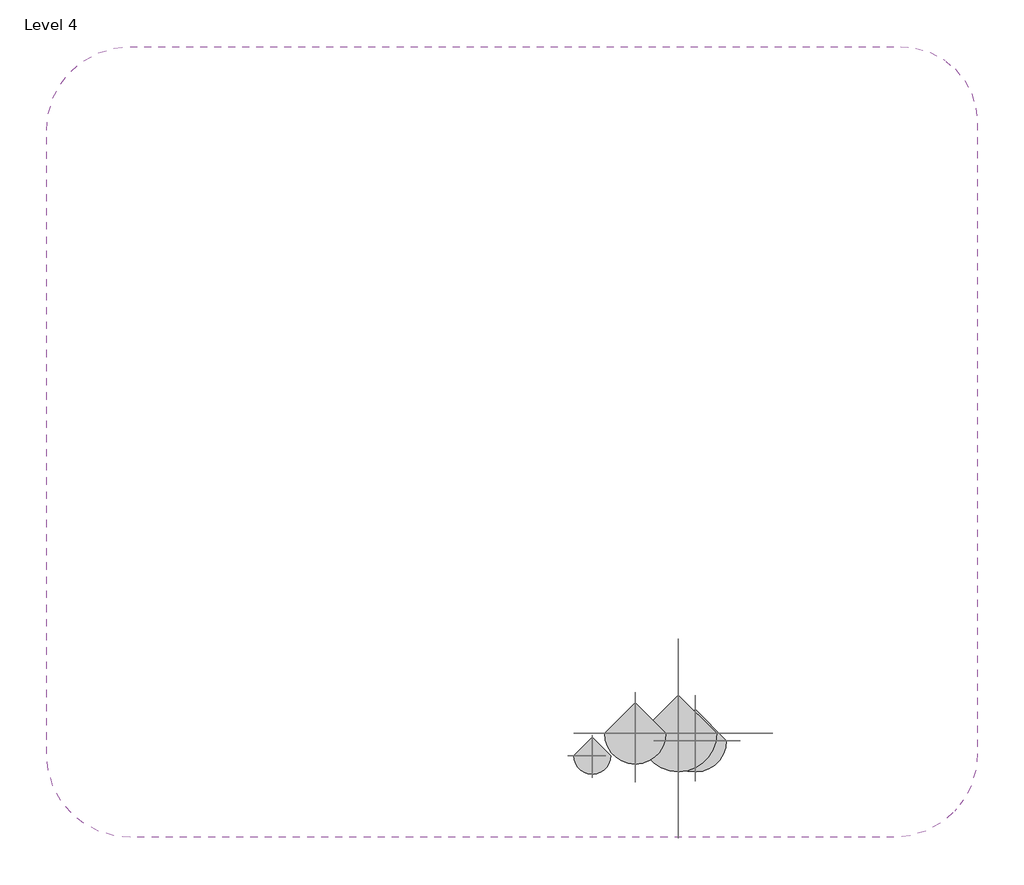
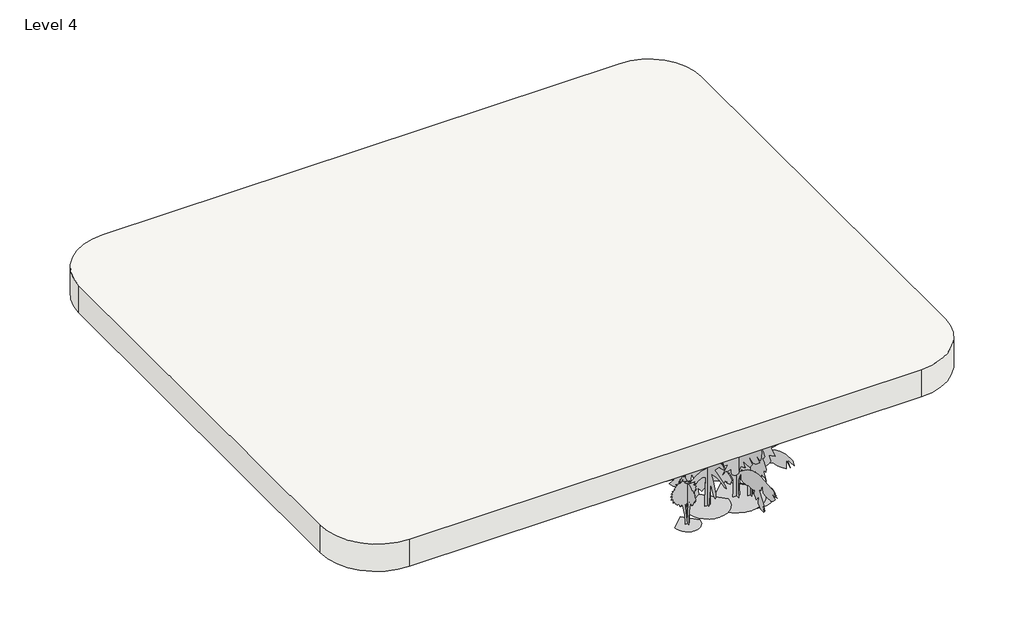
# One storey, incomplete: 4 geographic elements, 1 slab.
"""IFC4 building model written with IfcOpenShell, lengths in millimetres."""

from ifc_helpers import new_model, si_unit, point, frame, frame_2d, origin, place, context, project, spatial, polyline, circle_curve, trimmed, segment, composite_curve, outline, extrude, transform, mapped, element, save
from components import rpc_tree_tropical_82ff1ee0, rpc_tree_tropical_d7a905c7, rpc_tree_tropical_golden_malay_palm_10_a310d7cf, rpc_tree_tropical_japanese_fiber_banana_8_fc2fb2a9

model = new_model("IFC4")

# Units and contexts
model_context = context("Model", 3, world=origin())
ifc_project = project(units=[si_unit("LENGTHUNIT", "METRE", prefix="MILLI")], contexts=[model_context])

# Site, building, storey
site = spatial("IfcSite", under=ifc_project)
building = spatial("IfcBuilding", under=site)
storey = spatial("IfcBuildingStorey", under=building, Name="Level 4", Elevation=9144.0)

# Geographic elements
placement = place(None, origin())
rpc_tree_tropical_shape = rpc_tree_tropical_82ff1ee0(model_context)
element("IfcGeographicElement", 1, ObjectType="RPC Tree - Tropical", at=placement, inside=storey, context=model_context, shape_type="MappedRepresentation", body=[
    mapped(rpc_tree_tropical_shape, transform((-4130.1533244, -599.0997962, 7924.8), x_axis=(1.0, 0.0, 0.0), y_axis=(0.0, 1.0, 0.0), z_axis=(0.0, 0.0, 1.0))),
])
rpc_tree_tropical_2_shape = rpc_tree_tropical_d7a905c7(model_context)
element("IfcGeographicElement", 2, ObjectType="RPC Tree - Tropical", at=placement, inside=storey, context=model_context, shape_type="MappedRepresentation", body=[
    mapped(rpc_tree_tropical_2_shape, transform((-1945.7533244, -278.3567338, 7924.8), x_axis=(1.0, 0.0, 0.0), y_axis=(0.0, 1.0, 0.0), z_axis=(0.0, 0.0, 1.0))),
])
rpc_tree_tropical_golden_malay_palm_10_shape = rpc_tree_tropical_golden_malay_palm_10_a310d7cf(model_context)
element("IfcGeographicElement", 3, ObjectType="RPC Tree - Tropical : Golden Malay Palm - 10'", at=placement, inside=storey, context=model_context, shape_type="MappedRepresentation", body=[
    mapped(rpc_tree_tropical_golden_malay_palm_10_shape, transform((-2301.3533244, -125.9567338, 7924.8), x_axis=(1.0, 0.0, 0.0), y_axis=(0.0, 1.0, 0.0), z_axis=(0.0, 0.0, 1.0))),
])
rpc_tree_tropical_japanese_fiber_banana_8_shape = rpc_tree_tropical_japanese_fiber_banana_8_fc2fb2a9(model_context)
element("IfcGeographicElement", 4, ObjectType="RPC Tree - Tropical : Japanese Fiber Banana - 8'", at=placement, inside=storey, context=model_context, shape_type="MappedRepresentation", body=[
    mapped(rpc_tree_tropical_japanese_fiber_banana_8_shape, transform((-3215.7533244, -125.9567338, 7924.8), x_axis=(1.0, 0.0, 0.0), y_axis=(0.0, 1.0, 0.0), z_axis=(0.0, 0.0, 1.0))),
])

# Slab
element("IfcSlab", 5, ObjectType="Generic - 3'", at=placement, inside=storey, context=model_context, shape_type="SweptSolid", body=[
    extrude(outline(composite_curve([segment(trimmed(circle_curve(frame_2d((2423.0466756, 12828.0432662)), 1625.6), [point((2423.0466756, 14453.6432662))], [point((4048.6466756, 12828.0432662))], False, "CARTESIAN"), True, "CONTINUOUS"), segment(polyline([(4048.6466756, 12828.0432662), (4048.6466756, -557.7567338)]), True, "CONTINUOUS"), segment(trimmed(circle_curve(frame_2d((2270.6466756, -557.7567338)), 1778.0), [point((4048.6466756, -557.7567338))], [point((2270.6466756, -2335.7567338))], False, "CARTESIAN"), True, "CONTINUOUS"), segment(polyline([(2270.6466756, -2335.7567338), (-13934.5533244, -2335.7567338)]), True, "CONTINUOUS"), segment(trimmed(circle_curve(frame_2d((-13934.5533244, -557.7567338)), 1778.0), [point((-13934.5533244, -2335.7567338))], [point((-15712.5533244, -557.7567338))], False, "CARTESIAN"), True, "CONTINUOUS"), segment(polyline([(-15712.5533244, -557.7567338), (-15712.5533244, 12675.6432662)]), True, "CONTINUOUS"), segment(trimmed(circle_curve(frame_2d((-13934.5533244, 12675.6432662)), 1778.0), [point((-15712.5533244, 12675.6432662))], [point((-13934.5533244, 14453.6432662))], False, "CARTESIAN"), True, "CONTINUOUS"), segment(polyline([(-13934.5533244, 14453.6432662), (2423.0466756, 14453.6432662)]), True, "CONTINUOUS")], self_intersect=False)), frame((0.0, 0.0, 10979.15), z_axis=(0.0, 0.0, 1.0), x_axis=(1.0, 0.0, 0.0)), (0.0, 0.0, 1.0), 914.4),
])

save(model, "model.ifc")

# Revit data of these elements
# Type "RPC Tree - Tropical"
#   built-in parameter 1005198 = "{2, 15},{39, RPC-16-FXGL-GN00-PMD1-0000-ST1L-LVER-AU},{1, 0},{1, 0},{2, 13},{1, 8},{5, Color},{1, 0},{1, 0},{3, 0.8},{3, 0.8},{3, 0.8},{1, 8},{7, BBoxMin},{1, 0},{1, 0},{1, 0},{1, 0},{1, 0},{1, 8},{7, BBoxMax},{1, 0},{1, 0},{1, 0},{1, 0},{1, 0},{2, 11},{9, RPCTypeId},{1, 0},{1, 0},{39, RPC-16-FXGL-GN00-PMD1-0000-ST1L-LVER-AU},{1, 6},{14, RPCPlantHeight},{1, 0},{1, 0},{1, 5},{2, 11},{7, keyword},{1, 0},{1, 0},{35, :RPCs:Trees [Tropical]:Geometry:RPC},{2, 11},{8, category},{1, 0},{1, 0},{16, Trees [Tropical]},{2, 11},{12, LocalizedUID},{1, 0},{1, 0},{19, Buddha Belly Bamboo},{2, 14},{6, Height},{1, 0},{1, 0},{1, 5},{1, 2},{16, Cast Reflections},{1, 0},{1, 0},{1, 0},{1, 2},{12, Cast Shadows},{1, 0},{1, 0},{1, 1},{1, 2},{9, Lock View},{1, 0},{1, 0},{1, 0},{1, 4},{5, ViewC},{1, 0},{1, 0},{1, 0},{21, assetlibrary_base.fbx},{1, 5},"
#   built-in parameter 1005195 = "RPC-16-FXGL-GN00-PMD1-0000-ST1L-LVER-AU"
#   Assembly Code = "G2050500"
#   Height = 5' - 0"
#   Plan Symbol = element 361270
#   Default Elevation = 0
# Type "RPC Tree - Tropical"
#   built-in parameter 1005198 = "{2, 15},{39, RPC-16-G2MF-J1Q0-CAN1-N000-ST1L-LVER-AU},{1, 0},{1, 0},{2, 13},{1, 8},{5, Color},{1, 0},{1, 0},{3, 0.8},{3, 0.8},{3, 0.8},{1, 8},{7, BBoxMin},{1, 0},{1, 0},{1, 0},{1, 0},{1, 0},{1, 8},{7, BBoxMax},{1, 0},{1, 0},{1, 0},{1, 0},{1, 0},{2, 11},{9, RPCTypeId},{1, 0},{1, 0},{39, RPC-16-G2MF-J1Q0-CAN1-N000-ST1L-LVER-AU},{1, 6},{14, RPCPlantHeight},{1, 0},{1, 0},{1, 8},{2, 11},{7, keyword},{1, 0},{1, 0},{35, :RPCs:Trees [Tropical]:Geometry:RPC},{2, 11},{8, category},{1, 0},{1, 0},{16, Trees [Tropical]},{2, 11},{12, LocalizedUID},{1, 0},{1, 0},{13, Windmill Palm},{2, 14},{6, Height},{1, 0},{1, 0},{1, 8},{1, 2},{16, Cast Reflections},{1, 0},{1, 0},{1, 0},{1, 2},{12, Cast Shadows},{1, 0},{1, 0},{1, 1},{1, 2},{9, Lock View},{1, 0},{1, 0},{1, 0},{1, 4},{5, ViewC},{1, 0},{1, 0},{1, 0},{21, assetlibrary_base.fbx},{1, 5},"
#   built-in parameter 1005195 = "RPC-16-G2MF-J1Q0-CAN1-N000-ST1L-LVER-AU"
#   Assembly Code = "G2050500"
#   Height = 8' - 0"
#   Plan Symbol = element 361270
#   Default Elevation = 0
# Type "RPC Tree - Tropical : Golden Malay Palm - 10'"
#   built-in parameter 1005198 = "{2, 15},{39, RPC-16-FXGM-2RXX-PGXL-E000-ST1L-LVER-AU},{1, 0},{1, 0},{2, 13},{1, 8},{5, Color},{1, 0},{1, 0},{3, 0.8},{3, 0.8},{3, 0.8},{1, 8},{7, BBoxMin},{1, 0},{1, 0},{1, 0},{1, 0},{1, 0},{1, 8},{7, BBoxMax},{1, 0},{1, 0},{1, 0},{1, 0},{1, 0},{2, 11},{9, RPCTypeId},{1, 0},{1, 0},{39, RPC-16-FXGM-2RXX-PGXL-E000-ST1L-LVER-AU},{1, 6},{14, RPCPlantHeight},{1, 0},{1, 0},{2, 10},{2, 11},{7, keyword},{1, 0},{1, 0},{35, :RPCs:Trees [Tropical]:Geometry:RPC},{2, 11},{8, category},{1, 0},{1, 0},{16, Trees [Tropical]},{2, 11},{12, LocalizedUID},{1, 0},{1, 0},{17, Golden Malay Palm},{2, 14},{6, Height},{1, 0},{1, 0},{2, 10},{1, 2},{16, Cast Reflections},{1, 0},{1, 0},{1, 0},{1, 2},{12, Cast Shadows},{1, 0},{1, 0},{1, 1},{1, 2},{9, Lock View},{1, 0},{1, 0},{1, 0},{1, 4},{5, ViewC},{1, 0},{1, 0},{1, 0},{21, assetlibrary_base.fbx},{1, 5},"
#   built-in parameter 1005195 = "RPC-16-FXGM-2RXX-PGXL-E000-ST1L-LVER-AU"
#   Type Comments = "Golden Malay Palm"
#   Assembly Code = "G2050500"
#   Height = 10' - 0"
#   Plan Symbol = element 361270
#   Default Elevation = 0
# Type "RPC Tree - Tropical : Japanese Fiber Banana - 8'"
#   built-in parameter 1005198 = "{2, 15},{39, RPC-16-FVGT-NR7X-7G1M-A000-ST1L-LVER-AU},{1, 0},{1, 0},{2, 13},{1, 8},{5, Color},{1, 0},{1, 0},{3, 0.8},{3, 0.8},{3, 0.8},{1, 8},{7, BBoxMin},{1, 0},{1, 0},{1, 0},{1, 0},{1, 0},{1, 8},{7, BBoxMax},{1, 0},{1, 0},{1, 0},{1, 0},{1, 0},{2, 11},{9, RPCTypeId},{1, 0},{1, 0},{39, RPC-16-FVGT-NR7X-7G1M-A000-ST1L-LVER-AU},{1, 6},{14, RPCPlantHeight},{1, 0},{1, 0},{1, 8},{2, 11},{7, keyword},{1, 0},{1, 0},{35, :RPCs:Trees [Tropical]:Geometry:RPC},{2, 11},{8, category},{1, 0},{1, 0},{16, Trees [Tropical]},{2, 11},{12, LocalizedUID},{1, 0},{1, 0},{21, Japanese Fiber Banana},{2, 14},{6, Height},{1, 0},{1, 0},{1, 8},{1, 2},{16, Cast Reflections},{1, 0},{1, 0},{1, 0},{1, 2},{12, Cast Shadows},{1, 0},{1, 0},{1, 1},{1, 2},{9, Lock View},{1, 0},{1, 0},{1, 0},{1, 4},{5, ViewC},{1, 0},{1, 0},{1, 0},{21, assetlibrary_base.fbx},{1, 5},"
#   built-in parameter 1005195 = "RPC-16-FVGT-NR7X-7G1M-A000-ST1L-LVER-AU"
#   Type Comments = "Japanese Fiber Banana"
#   Assembly Code = "G2050500"
#   Height = 8' - 0"
#   Plan Symbol = element 361270
#   Default Elevation = 0
# Type "Generic - 3'"
#   Assembly Code = "B1010"
#   Function = 0
#   Layers, outside or top first: 3' - 0" "Cherry" (function 1)
# Elements 1, 2 (IfcGeographicElement, "RPC Tree - Tropical")
#   Phase Created = New Construction
# Element 3 (IfcGeographicElement, "RPC Tree - Tropical : Golden Malay Palm - 10'")
#   Phase Created = New Construction
# Element 4 (IfcGeographicElement, "RPC Tree - Tropical : Japanese Fiber Banana - 8'")
#   Phase Created = New Construction
# Element 5 (IfcSlab, "Generic - 3'")
#   Height Offset From Level = 9' - 0 1/4"
#   Phase Created = New Construction
#   Materials on its faces: "Cherry"
# Materials
#   "Cherry": class "Wood", colour RGB 238 208 179, transparency 0, Description = "Prunus Serotina", Cost = 0
